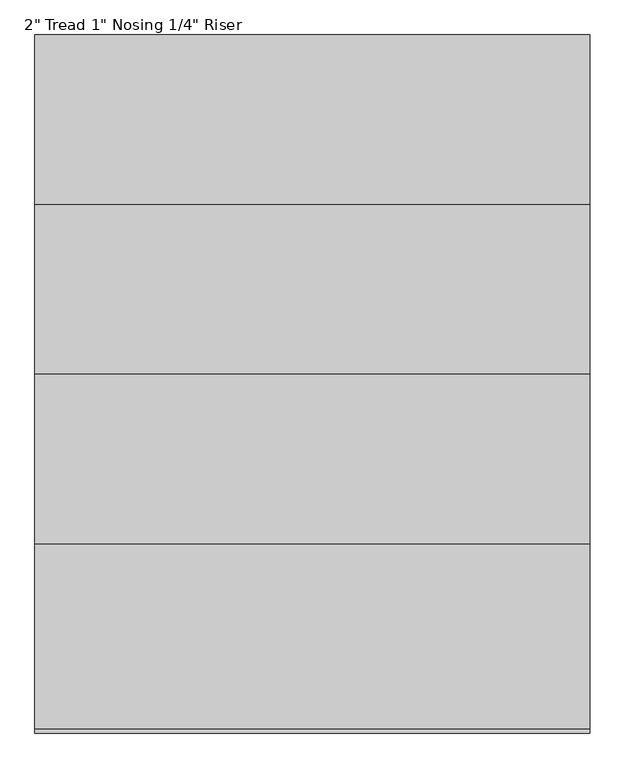
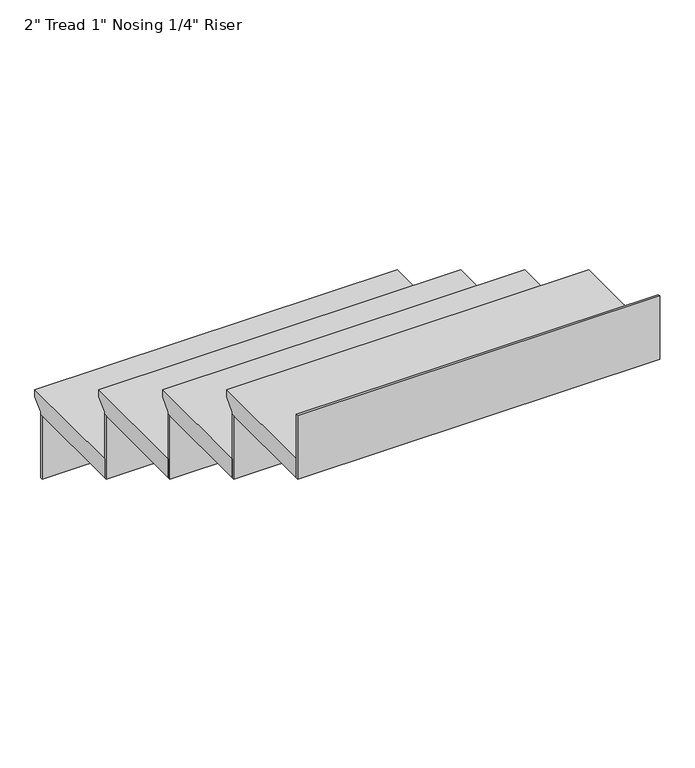
"""IFC4 building model written with IfcOpenShell, lengths in millimetres: stair flight geometry."""

from ifc_helpers import new_model, si_unit, frame, origin, place, context, project, spatial, polyline, outline, extrude, source, transform, mapped, element, save


def stair_flight_6e3cd39c(model_context):
    return source(origin(), model_context, "Body", "SweptSolid", [
        extrude(outline(polyline([(22889.9216096, 48941.2839133), (23194.7216096, 48941.2839133), (23194.7216096, 48922.2339133), (23169.3216096, 48896.8339133), (23169.3216096, 48890.4839133), (22889.9216096, 48890.4839133), (22889.9216096, 48941.2839133)])), frame((-2398.2415084, 0.0, 0.0), z_axis=(1.0, 0.0, 0.0), x_axis=(0.0, 1.0, 0.0)), (0.0, 0.0, 1.0), 914.4),
        extrude(outline(polyline([(-2398.2415084, 23162.9716096), (-2398.2415084, 23169.3216096), (-1483.8415084, 23169.3216096), (-1483.8415084, 23162.9716096), (-2398.2415084, 23162.9716096)])), frame((0.0, 0.0, 48721.1505799), z_axis=(0.0, 0.0, 1.0), x_axis=(1.0, 0.0, 0.0)), (0.0, 0.0, 1.0), 169.3333333),
        extrude(outline(polyline([(-2398.2415084, 22883.5716096), (-2398.2415084, 22889.9216096), (-1483.8415084, 22889.9216096), (-1483.8415084, 22883.5716096), (-2398.2415084, 22883.5716096)])), frame((0.0, 0.0, 48890.4839133), z_axis=(0.0, 0.0, 1.0), x_axis=(1.0, 0.0, 0.0)), (0.0, 0.0, 1.0), 169.3333333),
        extrude(outline(polyline([(22610.5216096, 49110.6172466), (22915.3216096, 49110.6172466), (22915.3216096, 49091.5672466), (22889.9216096, 49066.1672466), (22889.9216096, 49059.8172466), (22610.5216096, 49059.8172466), (22610.5216096, 49110.6172466)])), frame((-2398.2415084, 0.0, 0.0), z_axis=(1.0, 0.0, 0.0), x_axis=(0.0, 1.0, 0.0)), (0.0, 0.0, 1.0), 914.4),
        extrude(outline(polyline([(-2398.2415084, 22604.1716096), (-2398.2415084, 22610.5216096), (-1483.8415084, 22610.5216096), (-1483.8415084, 22604.1716096), (-2398.2415084, 22604.1716096)])), frame((0.0, 0.0, 49059.8172466), z_axis=(0.0, 0.0, 1.0), x_axis=(1.0, 0.0, 0.0)), (0.0, 0.0, 1.0), 169.3333333),
        extrude(outline(polyline([(22331.1216096, 49279.9505799), (22635.9216096, 49279.9505799), (22635.9216096, 49260.9005799), (22610.5216096, 49235.5005799), (22610.5216096, 49229.1505799), (22331.1216096, 49229.1505799), (22331.1216096, 49279.9505799)])), frame((-2398.2415084, 0.0, 0.0), z_axis=(1.0, 0.0, 0.0), x_axis=(0.0, 1.0, 0.0)), (0.0, 0.0, 1.0), 914.4),
        extrude(outline(polyline([(-2398.2415084, 22324.7716096), (-2398.2415084, 22331.1216096), (-1483.8415084, 22331.1216096), (-1483.8415084, 22324.7716096), (-2398.2415084, 22324.7716096)])), frame((0.0, 0.0, 49229.1505799), z_axis=(0.0, 0.0, 1.0), x_axis=(1.0, 0.0, 0.0)), (0.0, 0.0, 1.0), 169.3333333),
        extrude(outline(polyline([(-2398.2415084, 22045.3716096), (-2398.2415084, 22051.7216096), (-1483.8415084, 22051.7216096), (-1483.8415084, 22045.3716096), (-2398.2415084, 22045.3716096)])), frame((0.0, 0.0, 49398.4839133), z_axis=(0.0, 0.0, 1.0), x_axis=(1.0, 0.0, 0.0)), (0.0, 0.0, 1.0), 169.3333333),
        extrude(outline(polyline([(22051.7216096, 49449.2839133), (22356.5216096, 49449.2839133), (22356.5216096, 49430.2339133), (22331.1216096, 49404.8339133), (22331.1216096, 49398.4839133), (22051.7216096, 49398.4839133), (22051.7216096, 49449.2839133)])), frame((-2398.2415084, 0.0, 0.0), z_axis=(1.0, 0.0, 0.0), x_axis=(0.0, 1.0, 0.0)), (0.0, 0.0, 1.0), 914.4),
    ])


if __name__ == "__main__":
    model = new_model("IFC4")
    model_context = context("Model", 3, world=origin())
    ifc_project = project(units=[si_unit("LENGTHUNIT", "METRE", prefix="MILLI")], contexts=[model_context])
    site = spatial("IfcSite", under=ifc_project)
    building = spatial("IfcBuilding", under=site)
    placement = place(None, origin())
    stair_flight_shape = stair_flight_6e3cd39c(model_context)
    element("IfcStairFlight", 1, ObjectType="2\" Tread 1\" Nosing 1/4\" Riser", at=placement, inside=building, context=model_context, shape_type="MappedRepresentation", body=[
        mapped(stair_flight_shape, transform((0.0, 0.0, 0.0), x_axis=(1.0, 0.0, 0.0), y_axis=(0.0, 1.0, 0.0), z_axis=(0.0, 0.0, 1.0))),
    ])
    save(model, "model.ifc")
